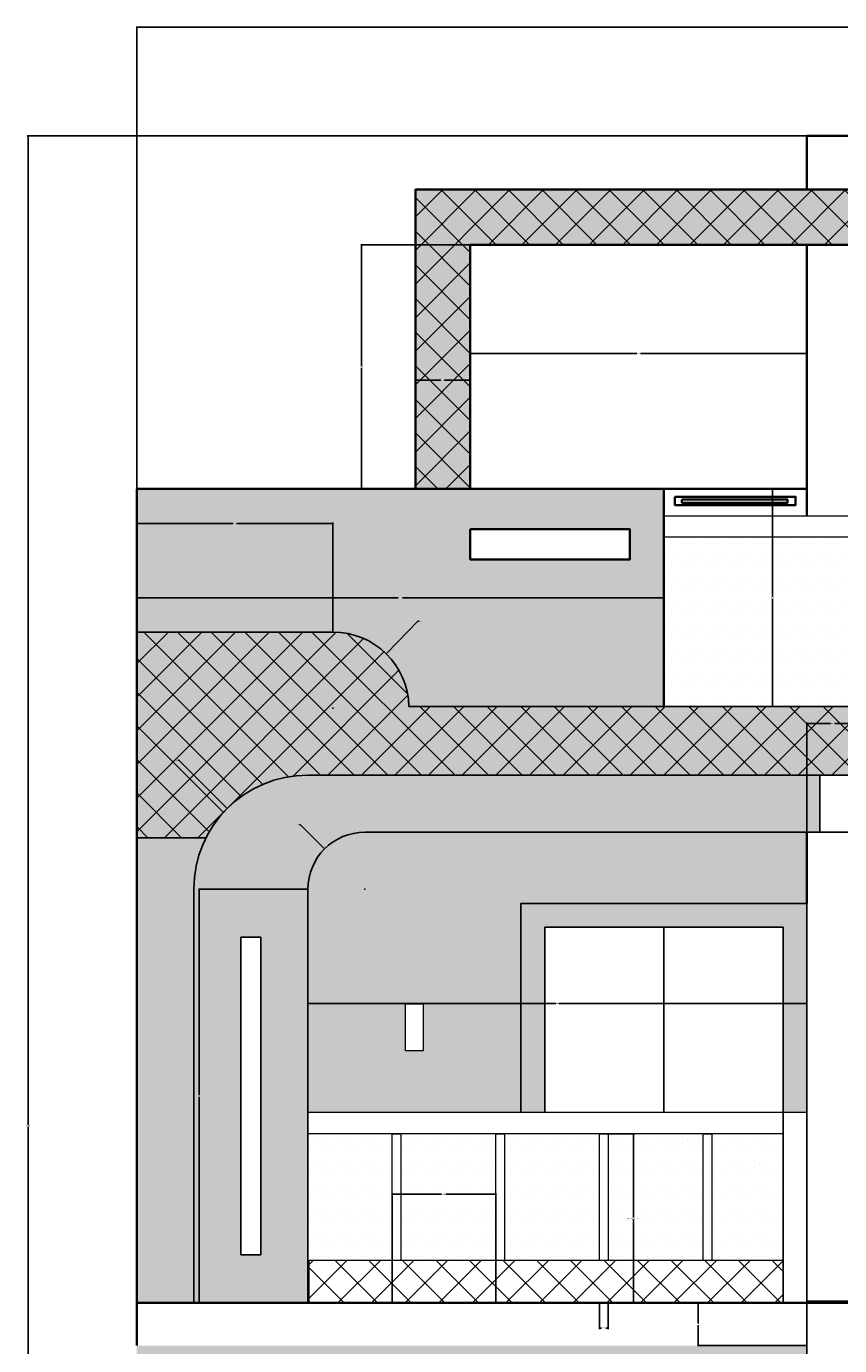
# Model space of a CAD drawing. Units: inches. Extents: x -13 to 333, y -76 to 399.
# Tile 2 of 3: x -13 to 158, y 121 to 399. Entities that reach past the tile are written whole.
import ezdxf

# ---------------------------------------------------------------- set-up
doc = ezdxf.new("R2010")
doc.units = ezdxf.units.IN
doc.header["$MEASUREMENT"] = 0
for name, color, linetype, lineweight in [('A-ANNO-DIMS', 2, 'Continuous', 18), ('A-DOOR', 3, 'Continuous', 25), ('A-ELEV-PATT', 252, 'Continuous', 13), ('A-ELEV-TRIM', 7, 'Continuous', 25), ('A-FLOR', 7, 'Continuous', 35), ('A-FLOR-HRAL', 4, 'Continuous', 20), ('A-FLOR-HRAL-PATT', 8, 'Continuous', 13), ('A-ROOF', 7, 'Continuous', 35), ('A-WALL', 7, 'Continuous', 35), ('A-WALL-PATT', 252, 'Continuous', 13), ('E-LITE-EXTR', 2, 'Continuous', 18)]:
    doc.layers.add(name, color=color, linetype=linetype, lineweight=lineweight)
doc.styles.get("Standard").update_dxf_attribs({"font": 'arial.ttf'})
doc.dimstyles.get("Standard").update_dxf_attribs({"dimtxt": 0.18, "dimasz": 0.18, "dimexe": 0.18, "dimexo": 0.0625, "dimgap": 0.09, "dimtad": 0, "dimtih": 1, "dimtoh": 1, "dimdec": 4, "dimzin": 0, "dimdsep": 46, "dimtxsty": 'Standard', "dimcen": 0.09, "dimadec": 0, "dimazin": 0, "dimtfac": 1, "dimtdec": 4, "dimtofl": 0, "dimtmove": 0, "dimatfit": 3, "dimfxl": 1, "dimtolj": 1, "dimtzin": 0, "dimarcsym": 0})

# ---------------------------------------------------------------- blocks, each defined once
blk = doc.blocks.new('LIGHT-WALL-SCONCE')
blk.add_lwpolyline([(0, 9.86), (3.7, 9.86), (3.7, 0), (0, 0)], close=True)
blk = doc.blocks.new('FASCIA-BATTEN')
blk.add_lwpolyline([(0, 12), (0, 0), (2.72, 0), (2.72, 12)])
blk = doc.blocks.new('GUARD-POST-BALCONY')
for points in [[(0, 9), (0, 35.57), (1.84, 35.57), (1.84, 9)], [(1.84, 0), (0, 0)]]:
    blk.add_lwpolyline(points)
blk = doc.blocks.new('*D12')
at = {"layer": 'A-ANNO-DIMS', "color": 0, "lineweight": -2, "transparency": 16777216}
for p, q in [((109.32, 165.75), (114.78, 165.75)), ((114.6, 165.57), (114.6, 148.15)), ((114.6, 130.36), (114.6, 147.78)), ((109.32, 130.18), (114.78, 130.18))]:
    blk.add_line(p, q, dxfattribs=at)
at = {"layer": 'A-ANNO-DIMS', "color": 0, "transparency": 16777216}
for points in [[(114.57, 165.57), (114.63, 165.57), (114.6, 165.75)], [(114.57, 130.36), (114.63, 130.36), (114.6, 130.18)]]:
    blk.add_solid(points, dxfattribs=at)
at = {"layer": 'Defpoints', "color": 0, "transparency": 16777216}
for p in [(109.26, 165.75), (114.6, 165.75), (109.26, 130.18)]:
    blk.add_point(p, dxfattribs=at)
at = {"layer": 'A-ANNO-DIMS', "color": 0, "transparency": 16777216, "insert": (114.6, 147.96), "char_height": 0.18, "attachment_point": 5}
blk.add_mtext('\\A1;BALCONY POST 36 TYP.', dxfattribs=at)
blk = doc.blocks.new('*D13')
at = {"layer": 'A-ANNO-DIMS', "color": 0, "lineweight": -2, "transparency": 16777216}
for p, q in [((107.42, 130.11), (107.42, 124.66)), ((109.26, 130.11), (109.26, 124.66)), ((107.6, 124.84), (107.88, 124.84)), ((109.08, 124.84), (108.8, 124.84))]:
    blk.add_line(p, q, dxfattribs=at)
at = {"layer": 'A-ANNO-DIMS', "color": 0, "transparency": 16777216}
for points in [[(107.6, 124.87), (107.6, 124.81), (107.42, 124.84)], [(109.08, 124.87), (109.08, 124.81), (109.26, 124.84)]]:
    blk.add_solid(points, dxfattribs=at)
at = {"layer": 'Defpoints', "color": 0, "transparency": 16777216}
for p in [(107.42, 130.18), (109.26, 130.18), (109.26, 124.84)]:
    blk.add_point(p, dxfattribs=at)
at = {"layer": 'A-ANNO-DIMS', "color": 0, "transparency": 16777216, "insert": (108.34, 124.84), "char_height": 0.18, "attachment_point": 5}
blk.add_mtext('\\A1;2 TYP.', dxfattribs=at)
blk = doc.blocks.new('*D16')
at = {"layer": 'A-ANNO-DIMS', "color": 0, "lineweight": -2, "transparency": 16777216}
for p, q in [((10.07, 301.43), (10.07, 398.67)), ((10.25, 398.49), (159.78, 398.49)), ((309.89, 398.49), (160.36, 398.49)), ((310.07, 375.69), (310.07, 398.67))]:
    blk.add_line(p, q, dxfattribs=at)
at = {"layer": 'A-ANNO-DIMS', "color": 0, "transparency": 16777216}
for points in [[(10.25, 398.52), (10.25, 398.46), (10.07, 398.49)], [(309.89, 398.52), (309.89, 398.46), (310.07, 398.49)]]:
    blk.add_solid(points, dxfattribs=at)
at = {"layer": 'Defpoints', "color": 0, "transparency": 16777216}
for p in [(310.07, 398.49), (310.07, 375.63), (10.07, 301.36)]:
    blk.add_point(p, dxfattribs=at)
at = {"layer": 'A-ANNO-DIMS', "color": 0, "transparency": 16777216, "insert": (160.07, 398.49), "char_height": 0.18, "attachment_point": 5}
blk.add_mtext('\\A1;300', dxfattribs=at)
blk = doc.blocks.new('*D17')
at = {"layer": 'A-ANNO-DIMS', "color": 0, "lineweight": -2, "transparency": 16777216}
for p, q in [((151.01, 375.63), (-12.97, 375.63)), ((-12.79, 375.45), (-12.79, 167.59)), ((-12.79, -40.64), (-12.79, 167.22)), ((10.01, -40.82), (-12.97, -40.82))]:
    blk.add_line(p, q, dxfattribs=at)
at = {"layer": 'A-ANNO-DIMS', "color": 0, "transparency": 16777216}
for points in [[(-12.82, 375.45), (-12.76, 375.45), (-12.79, 375.63)], [(-12.82, -40.64), (-12.76, -40.64), (-12.79, -40.82)]]:
    blk.add_solid(points, dxfattribs=at)
at = {"layer": 'Defpoints', "color": 0, "transparency": 16777216}
for p in [(-12.79, 375.63), (151.07, 375.63), (10.07, -40.82)]:
    blk.add_point(p, dxfattribs=at)
at = {"layer": 'A-ANNO-DIMS', "color": 0, "transparency": 16777216, "insert": (-12.79, 167.4), "char_height": 0.18, "attachment_point": 5}
blk.add_mtext('\\A1;416.46', dxfattribs=at)
blk = doc.blocks.new('*D33')
at = {"layer": 'A-ANNO-DIMS', "color": 0, "lineweight": -2, "transparency": 16777216}
for p, q in [((46.01, 217.18), (23.03, 217.18)), ((23.21, 217), (23.21, 173.86)), ((23.21, 130.36), (23.21, 173.49)), ((46.01, 130.18), (23.03, 130.18))]:
    blk.add_line(p, q, dxfattribs=at)
at = {"layer": 'A-ANNO-DIMS', "color": 0, "transparency": 16777216}
for points in [[(23.18, 217), (23.24, 217), (23.21, 217.18)], [(23.18, 130.36), (23.24, 130.36), (23.21, 130.18)]]:
    blk.add_solid(points, dxfattribs=at)
at = {"layer": 'Defpoints', "color": 0, "transparency": 16777216}
for p in [(23.21, 217.18), (46.07, 217.18), (46.07, 130.18)]:
    blk.add_point(p, dxfattribs=at)
at = {"layer": 'A-ANNO-DIMS', "color": 0, "transparency": 16777216, "insert": (23.21, 173.68), "char_height": 0.18, "attachment_point": 5}
blk.add_mtext('\\A1;87', dxfattribs=at)
blk = doc.blocks.new('*D34')
at = {"layer": 'A-ANNO-DIMS', "color": 0, "lineweight": -2, "transparency": 16777216}
for p, q in [((63.78, 130.24), (63.78, 153.22)), ((63.96, 153.04), (74.22, 153.04)), ((85.42, 153.04), (75.15, 153.04)), ((85.6, 130.24), (85.6, 153.22))]:
    blk.add_line(p, q, dxfattribs=at)
at = {"layer": 'A-ANNO-DIMS', "color": 0, "transparency": 16777216}
for points in [[(63.96, 153.07), (63.96, 153.01), (63.78, 153.04)], [(85.42, 153.07), (85.42, 153.01), (85.6, 153.04)]]:
    blk.add_solid(points, dxfattribs=at)
at = {"layer": 'Defpoints', "color": 0, "transparency": 16777216}
for p in [(85.6, 153.04), (63.78, 130.18), (85.6, 130.18)]:
    blk.add_point(p, dxfattribs=at)
at = {"layer": 'A-ANNO-DIMS', "color": 0, "transparency": 16777216, "insert": (74.69, 153.04), "char_height": 0.18, "attachment_point": 5}
blk.add_mtext('\\A1;21.823', dxfattribs=at)
blk = doc.blocks.new('*D36')
at = {"layer": 'A-ANNO-DIMS', "color": 0, "lineweight": -2, "transparency": 16777216}
for p, q in [((151.07, 229.24), (151.07, 252.22)), ((151.25, 252.04), (156.06, 252.04)), ((161.78, 252.04), (156.97, 252.04)), ((161.96, 229.24), (161.96, 252.22))]:
    blk.add_line(p, q, dxfattribs=at)
at = {"layer": 'A-ANNO-DIMS', "color": 0, "transparency": 16777216}
for points in [[(151.25, 252.07), (151.25, 252.01), (151.07, 252.04)], [(161.78, 252.07), (161.78, 252.01), (161.96, 252.04)]]:
    blk.add_solid(points, dxfattribs=at)
at = {"layer": 'Defpoints', "color": 0, "transparency": 16777216}
for p in [(161.96, 252.04), (151.07, 229.18), (161.96, 229.18)]:
    blk.add_point(p, dxfattribs=at)
at = {"layer": 'A-ANNO-DIMS', "color": 0, "transparency": 16777216, "insert": (156.51, 252.04), "char_height": 0.18, "attachment_point": 5}
blk.add_mtext('\\A1;10.885', dxfattribs=at)
blk = doc.blocks.new('*D37')
at = {"layer": 'A-ANNO-DIMS', "color": 0, "lineweight": -2, "transparency": 16777216}
for p, q in [((121.05, 301.36), (144.03, 301.36)), ((143.85, 301.18), (143.85, 278.68)), ((143.85, 255.81), (143.85, 278.32)), ((121.05, 255.63), (144.03, 255.63))]:
    blk.add_line(p, q, dxfattribs=at)
at = {"layer": 'A-ANNO-DIMS', "color": 0, "transparency": 16777216}
for points in [[(143.82, 301.18), (143.88, 301.18), (143.85, 301.36)], [(143.82, 255.81), (143.88, 255.81), (143.85, 255.63)]]:
    blk.add_solid(points, dxfattribs=at)
at = {"layer": 'Defpoints', "color": 0, "transparency": 16777216}
for p in [(120.99, 301.36), (120.99, 255.63), (143.85, 255.63)]:
    blk.add_point(p, dxfattribs=at)
at = {"layer": 'A-ANNO-DIMS', "color": 0, "transparency": 16777216, "insert": (143.85, 278.5), "char_height": 0.18, "attachment_point": 5}
blk.add_mtext('\\A1;45.73', dxfattribs=at)
blk = doc.blocks.new('*D38')
at = {"layer": 'A-ANNO-DIMS', "color": 0, "lineweight": -2, "transparency": 16777216}
for p, q in [((10.07, 301.3), (10.07, 278.32)), ((120.99, 301.3), (120.99, 278.32)), ((10.25, 278.5), (65.08, 278.5)), ((120.81, 278.5), (65.98, 278.5))]:
    blk.add_line(p, q, dxfattribs=at)
at = {"layer": 'A-ANNO-DIMS', "color": 0, "transparency": 16777216}
for points in [[(10.25, 278.53), (10.25, 278.47), (10.07, 278.5)], [(120.81, 278.53), (120.81, 278.47), (120.99, 278.5)]]:
    blk.add_solid(points, dxfattribs=at)
at = {"layer": 'Defpoints', "color": 0, "transparency": 16777216}
for p in [(10.07, 301.36), (120.99, 301.36), (10.07, 278.5)]:
    blk.add_point(p, dxfattribs=at)
at = {"layer": 'A-ANNO-DIMS', "color": 0, "transparency": 16777216, "insert": (65.53, 278.5), "char_height": 0.18, "attachment_point": 5}
blk.add_mtext('\\A1;110.92', dxfattribs=at)
blk = doc.blocks.new('*D39')
at = {"layer": 'A-ANNO-DIMS', "color": 0, "lineweight": -2, "transparency": 16777216}
for p, q in [((80.24, 352.68), (80.24, 329.71)), ((151.07, 352.68), (151.07, 329.71)), ((80.42, 329.89), (115.26, 329.89)), ((150.89, 329.89), (116.05, 329.89))]:
    blk.add_line(p, q, dxfattribs=at)
at = {"layer": 'A-ANNO-DIMS', "color": 0, "transparency": 16777216}
for points in [[(80.42, 329.92), (80.42, 329.86), (80.24, 329.89)], [(150.89, 329.92), (150.89, 329.86), (151.07, 329.89)]]:
    blk.add_solid(points, dxfattribs=at)
at = {"layer": 'Defpoints', "color": 0, "transparency": 16777216}
for p in [(80.24, 352.75), (151.07, 352.75), (80.24, 329.89)]:
    blk.add_point(p, dxfattribs=at)
at = {"layer": 'A-ANNO-DIMS', "color": 0, "transparency": 16777216, "insert": (115.65, 329.89), "char_height": 0.18, "attachment_point": 5}
blk.add_mtext('\\A1;70.83', dxfattribs=at)
blk = doc.blocks.new('*D40')
at = {"layer": 'A-ANNO-DIMS', "color": 0, "lineweight": -2, "transparency": 16777216}
for p, q in [((80.18, 352.75), (57.2, 352.75)), ((57.38, 352.57), (57.38, 327.24)), ((57.38, 301.54), (57.38, 326.87)), ((80.18, 301.36), (57.2, 301.36))]:
    blk.add_line(p, q, dxfattribs=at)
at = {"layer": 'A-ANNO-DIMS', "color": 0, "transparency": 16777216}
for points in [[(57.35, 352.57), (57.41, 352.57), (57.38, 352.75)], [(57.35, 301.54), (57.41, 301.54), (57.38, 301.36)]]:
    blk.add_solid(points, dxfattribs=at)
at = {"layer": 'Defpoints', "color": 0, "transparency": 16777216}
for p in [(57.38, 352.75), (80.24, 352.75), (80.24, 301.36)]:
    blk.add_point(p, dxfattribs=at)
at = {"layer": 'A-ANNO-DIMS', "color": 0, "transparency": 16777216, "insert": (57.38, 327.05), "char_height": 0.18, "attachment_point": 5}
blk.add_mtext('\\A1;51.38', dxfattribs=at)
blk = doc.blocks.new('*D42')
at = {"layer": 'A-ANNO-DIMS', "color": 0, "lineweight": -2, "transparency": 16777216}
for p, q in [((46.07, 170.33), (46.07, 193.31)), ((46.25, 193.13), (98.29, 193.13)), ((150.89, 193.13), (98.85, 193.13)), ((151.07, 170.33), (151.07, 193.31))]:
    blk.add_line(p, q, dxfattribs=at)
at = {"layer": 'A-ANNO-DIMS', "color": 0, "transparency": 16777216}
for points in [[(46.25, 193.16), (46.25, 193.1), (46.07, 193.13)], [(150.89, 193.16), (150.89, 193.1), (151.07, 193.13)]]:
    blk.add_solid(points, dxfattribs=at)
at = {"layer": 'Defpoints', "color": 0, "transparency": 16777216}
for p in [(151.07, 193.13), (46.07, 170.27), (151.07, 170.27)]:
    blk.add_point(p, dxfattribs=at)
at = {"layer": 'A-ANNO-DIMS', "color": 0, "transparency": 16777216, "insert": (98.57, 193.13), "char_height": 0.18, "attachment_point": 5}
blk.add_mtext('\\A1;105', dxfattribs=at)
blk = doc.blocks.new('*D43')
at = {"layer": 'A-ANNO-DIMS', "color": 0, "lineweight": -2, "transparency": 16777216}
for p, q in [((151.07, 130.11), (151.07, 107.14)), ((172.62, 130.11), (172.62, 107.14)), ((151.25, 107.32), (161.38, 107.32)), ((172.44, 107.32), (162.31, 107.32))]:
    blk.add_line(p, q, dxfattribs=at)
at = {"layer": 'A-ANNO-DIMS', "color": 0, "transparency": 16777216}
for points in [[(151.25, 107.35), (151.25, 107.29), (151.07, 107.32)], [(172.44, 107.35), (172.44, 107.29), (172.62, 107.32)]]:
    blk.add_solid(points, dxfattribs=at)
at = {"layer": 'Defpoints', "color": 0, "transparency": 16777216}
for p in [(151.07, 130.18), (172.62, 130.18), (151.07, 107.32)]:
    blk.add_point(p, dxfattribs=at)
at = {"layer": 'A-ANNO-DIMS', "color": 0, "transparency": 16777216, "insert": (161.84, 107.32), "char_height": 0.18, "attachment_point": 5}
blk.add_mtext('\\A1;21.545', dxfattribs=at)
blk = doc.blocks.new('*D46')
at = {"layer": 'A-ANNO-DIMS', "color": 0, "lineweight": -2, "transparency": 16777216}
for p, q in [((151.01, 130.18), (128.03, 130.18)), ((128.21, 130), (128.21, 125.86)), ((128.21, 121.36), (128.21, 125.49)), ((151.01, 121.18), (128.03, 121.18))]:
    blk.add_line(p, q, dxfattribs=at)
at = {"layer": 'A-ANNO-DIMS', "color": 0, "transparency": 16777216}
for points in [[(128.18, 130), (128.24, 130), (128.21, 130.18)], [(128.18, 121.36), (128.24, 121.36), (128.21, 121.18)]]:
    blk.add_solid(points, dxfattribs=at)
at = {"layer": 'Defpoints', "color": 0, "transparency": 16777216}
for p in [(128.21, 130.18), (151.07, 130.18), (151.07, 121.18)]:
    blk.add_point(p, dxfattribs=at)
at = {"layer": 'A-ANNO-DIMS', "color": 0, "transparency": 16777216, "insert": (128.21, 125.68), "char_height": 0.18, "attachment_point": 5}
blk.add_mtext('\\A1;9', dxfattribs=at)
blk = doc.blocks.new('*D47')
at = {"layer": 'A-ANNO-DIMS', "color": 0, "lineweight": -2, "transparency": 16777216}
for p, q in [((68.7, 301.43), (68.7, 324.4)), ((68.88, 324.22), (74.08, 324.22)), ((80.06, 324.22), (74.85, 324.22)), ((80.24, 301.43), (80.24, 324.4))]:
    blk.add_line(p, q, dxfattribs=at)
at = {"layer": 'A-ANNO-DIMS', "color": 0, "transparency": 16777216}
for points in [[(68.88, 324.25), (68.88, 324.19), (68.7, 324.22)], [(80.06, 324.25), (80.06, 324.19), (80.24, 324.22)]]:
    blk.add_solid(points, dxfattribs=at)
at = {"layer": 'Defpoints', "color": 0, "transparency": 16777216}
for p in [(80.24, 324.22), (68.7, 301.36), (80.24, 301.36)]:
    blk.add_point(p, dxfattribs=at)
at = {"layer": 'A-ANNO-DIMS', "color": 0, "transparency": 16777216, "insert": (74.47, 324.22), "char_height": 0.18, "attachment_point": 5}
blk.add_mtext('\\A1;11.54', dxfattribs=at)
blk = doc.blocks.new('*D50')
at = {"layer": 'A-ANNO-DIMS', "color": 0, "lineweight": -2, "transparency": 16777216}
for p, q in [((10.07, 271.33), (10.07, 294.31)), ((51.35, 271.33), (51.35, 294.31)), ((10.25, 294.13), (30.31, 294.13)), ((51.17, 294.13), (31.11, 294.13))]:
    blk.add_line(p, q, dxfattribs=at)
at = {"layer": 'A-ANNO-DIMS', "color": 0, "transparency": 16777216}
for points in [[(10.25, 294.16), (10.25, 294.1), (10.07, 294.13)], [(51.17, 294.16), (51.17, 294.1), (51.35, 294.13)]]:
    blk.add_solid(points, dxfattribs=at)
at = {"layer": 'Defpoints', "color": 0, "transparency": 16777216}
for p in [(51.35, 294.13), (10.07, 271.27), (51.35, 271.27)]:
    blk.add_point(p, dxfattribs=at)
at = {"layer": 'A-ANNO-DIMS', "color": 0, "transparency": 16777216, "insert": (30.71, 294.13), "char_height": 0.18, "attachment_point": 5}
blk.add_mtext('\\A1;41.28', dxfattribs=at)
blk = doc.blocks.new('*D51')
at = {"layer": 'A-ANNO-DIMS', "color": 0, "lineweight": -2, "transparency": 16777216}
for p, q in [((18.74, 244.33), (18.92, 244.33)), ((18.92, 244.33), (28.97, 234.27)), ((45.98, 217.18), (46.16, 217.18)), ((46.07, 217.09), (46.07, 217.27))]:
    blk.add_line(p, q, dxfattribs=at)
at = {"layer": 'A-ANNO-DIMS', "color": 0, "transparency": 16777216}
blk.add_solid([(28.99, 234.29), (28.95, 234.25), (29.1, 234.15)], dxfattribs=at)
at = {"layer": 'Defpoints', "color": 0, "transparency": 16777216}
for p in [(29.1, 234.15), (46.07, 217.18)]:
    blk.add_point(p, dxfattribs=at)
at = {"layer": 'A-ANNO-DIMS', "color": 0, "transparency": 16777216, "insert": (18.43, 244.33), "char_height": 0.18, "attachment_point": 5}
blk.add_mtext('\\A1;R24', dxfattribs=at)
blk = doc.blocks.new('*D52')
at = {"layer": 'A-ANNO-DIMS', "color": 0, "lineweight": -2, "transparency": 16777216}
for p, q in [((69.24, 273.57), (62.66, 266.84)), ((69.42, 273.57), (69.24, 273.57)), ((51.35, 255.18), (51.35, 255.36)), ((51.26, 255.27), (51.44, 255.27))]:
    blk.add_line(p, q, dxfattribs=at)
at = {"layer": 'A-ANNO-DIMS', "color": 0, "transparency": 16777216}
blk.add_solid([(62.64, 266.86), (62.68, 266.82), (62.53, 266.71)], dxfattribs=at)
at = {"layer": 'Defpoints', "color": 0, "transparency": 16777216}
for p in [(62.53, 266.71), (51.35, 255.27)]:
    blk.add_point(p, dxfattribs=at)
at = {"layer": 'A-ANNO-DIMS', "color": 0, "transparency": 16777216, "insert": (69.73, 273.57), "char_height": 0.18, "attachment_point": 5}
blk.add_mtext('\\A1;R16', dxfattribs=at)
blk = doc.blocks.new('*D53')
at = {"layer": 'A-ANNO-DIMS', "color": 0, "lineweight": -2, "transparency": 16777216}
for p, q in [((44.31, 230.75), (44.49, 230.75)), ((44.49, 230.75), (49.46, 225.79)), ((57.98, 217.18), (58.16, 217.18)), ((58.07, 217.09), (58.07, 217.27))]:
    blk.add_line(p, q, dxfattribs=at)
at = {"layer": 'A-ANNO-DIMS', "color": 0, "transparency": 16777216}
blk.add_solid([(49.48, 225.81), (49.44, 225.77), (49.59, 225.66)], dxfattribs=at)
at = {"layer": 'Defpoints', "color": 0, "transparency": 16777216}
for p in [(49.59, 225.66), (58.07, 217.18)]:
    blk.add_point(p, dxfattribs=at)
at = {"layer": 'A-ANNO-DIMS', "color": 0, "transparency": 16777216, "insert": (44.01, 230.75), "char_height": 0.18, "attachment_point": 5}
blk.add_mtext('\\A1;R12', dxfattribs=at)

msp = doc.modelspace()

# ---------------------------------------------------------------- hatches: boundary and pattern name
at = {"layer": 'A-ELEV-PATT', "transparency": 33554595}
h = msp.add_hatch(color=256, dxfattribs=at)
h.dxf.hatch_style = 1
h.set_gradient(color1=(153, 27, 30), color2=(153, 27, 30))
h.paths.add_polyline_path([(151.0707, 214.1758), (90.9079, 214.1758), (90.9079, 170.2685), (95.9079, 170.2685), (95.9079, 209.1758), (146.0707, 209.1758), (146.0707, 170.2685), (151.0707, 170.2685)])
h.paths.add_polyline_path([(151.0707, 85.1758), (90.9079, 85.1758), (90.9079, 1.1758), (95.9079, 1.1758), (95.9079, 80.1758), (146.0707, 80.1758), (146.0707, 1.1758), (151.0707, 1.1758)])
h.paths.add_polyline_path([(60.8562, 85.1758), (27.7326, 85.1758), (27.7326, 37.5603), (60.8562, 37.5603)])
h.paths.add_polyline_path([(57.8562, 82.1758), (57.8562, 40.5603), (44.2944, 40.5603), (44.2944, 82.1758)], flags=16)
h.paths.add_polyline_path([(42.6571, 82.1758), (42.6571, 40.5603), (30.7326, 40.5603), (30.7326, 82.1758)], flags=16)
at = {"layer": 'A-FLOR-HRAL-PATT'}
h = msp.add_hatch(dxfattribs=at)
h.set_pattern_fill('DOTS', color=256, scale=40, style=0)
h.paths.add_polyline_path([(120.9893, 255.6309), (161.426, 255.6309), (161.426, 291.2047), (120.9893, 291.2047)])
h.paths.add_polyline_path([(163.2631, 255.6309), (203.6999, 255.6309), (203.6999, 291.2047), (163.2631, 291.2047)], flags=0)
h.paths.add_polyline_path([(205.537, 255.6309), (245.9737, 255.6309), (245.9737, 291.2047), (205.537, 291.2047)], flags=0)
h.paths.add_polyline_path([(247.8108, 255.6309), (288.2475, 255.6309), (288.2475, 291.2047), (247.8108, 291.2047)], flags=0)
h.paths.add_polyline_path([(290.0846, 255.6309), (310.0707, 255.6309), (310.0707, 291.2047), (290.0846, 291.2047)], flags=0)
at = {"layer": 'A-FLOR-HRAL-PATT', "transparency": 33554595}
h = msp.add_hatch(dxfattribs=at)
h.set_pattern_fill('DOTS', color=256, scale=40)
h.paths.add_polyline_path([(63.778, 165.7496), (46.0707, 165.7496), (46.0707, 130.1758), (46.3341, 130.1758), (46.3341, 139.1758), (63.778, 139.1758)])
h.paths.add_polyline_path([(85.6012, 165.7496), (65.6151, 165.7496), (65.6151, 139.1758), (85.6012, 139.1758)])
h.paths.add_polyline_path([(107.4244, 165.7496), (87.4383, 165.7496), (87.4383, 139.1758), (107.4244, 139.1758)])
h.paths.add_polyline_path([(129.2475, 165.7496), (109.2615, 165.7496), (109.2615, 139.1758), (129.2475, 139.1758)])
h.paths.add_polyline_path([(146.0707, 165.7496), (131.0846, 165.7496), (131.0846, 139.1758), (146.0707, 139.1758)])
at = {"layer": 'A-FLOR-HRAL-PATT', "transparency": 33554544}
h = msp.add_hatch(dxfattribs=at)
h.set_pattern_fill('ANSI37', color=256, scale=40)
h.paths.add_polyline_path([(146.0707, 139.1758), (46.3341, 139.1758), (46.3341, 130.1758), (146.0707, 130.1758)])
at = {"layer": 'A-WALL-PATT', "transparency": 33554556}
h = msp.add_hatch(dxfattribs=at)
h.set_pattern_fill('ANSI37', color=256, scale=40)
h.paths.add_polyline_path([(51.3479, 271.2697), (10.0707, 271.2697), (10.0707, 241.1758), (10.0707, 228.0051), (24.6528, 228.0051, -0.28286751), (46.0707, 241.1758), (310.0707, 241.1758), (310.0707, 255.6309), (67.3439, 255.6309, 0.40761741)])
h.paths.add_polyline_path([(80.2381, 352.7454), (310.0707, 352.7454), (310.0707, 364.3576), (80.2381, 364.3576), (68.6976, 364.3576), (68.6976, 301.3637), (80.2381, 301.3637)])
at = {"layer": 'A-WALL-PATT', "transparency": 33554595}
h = msp.add_hatch(color=256, dxfattribs=at)
h.dxf.hatch_style = 1
h.set_gradient(color1=(175, 217, 170), color2=(175, 217, 170))
h.paths.add_polyline_path([(310.0707, 364.3576), (80.2381, 364.3576), (68.6976, 364.3576), (68.6976, 301.3637), (80.2381, 301.3637), (80.2381, 352.7454), (310.0707, 352.7454)])
h.paths.add_polyline_path([(51.3479, 271.2697), (10.0707, 271.2697), (10.0707, 241.1758), (10.0707, 228.0051), (24.6528, 228.0051, -0.28286751), (46.0707, 241.1758), (310.0707, 241.1758), (310.0707, 255.6309), (67.3439, 255.6309, 0.40761741)])
h = msp.add_hatch(color=256, dxfattribs=at)
h.dxf.hatch_style = 1
h.set_gradient(color1=(229, 232, 120), color2=(200, 201, 45), name='INVHEMISPHERICAL')
h.paths.add_polyline_path([(120.9893, 301.3637), (10.0707, 301.3637), (10.0707, 271.2697), (51.3479, 271.2697, -0.40761741), (67.3439, 255.6309), (120.9893, 255.6309)])
h.paths.add_polyline_path([(80.2381, 286.5642), (80.2381, 292.8788), (113.8366, 292.8788), (113.8366, 286.5642)], flags=16)
h = msp.add_hatch(color=256, dxfattribs=at)
h.dxf.hatch_style = 1
h.set_gradient(color1=(39, 118, 187), color2=(39, 118, 187), name='INVSPHERICAL')
h.paths.add_polyline_path([(58.0707, 229.1758), (151.0707, 229.1758), (151.0707, 241.1758), (46.0707, 241.1758, 0.41421356), (22.0707, 217.1758), (22.0707, 130.1758), (46.0707, 130.1758), (46.0707, 217.1758, -0.41421356)])
h.paths.add_polyline_path([(36.1477, 207.0573), (36.1477, 140.2942), (31.9937, 140.2942), (31.9937, 207.0573)], flags=16)
at = {"layer": 'A-WALL-PATT', "transparency": 33554531}
h = msp.add_hatch(color=256, dxfattribs=at)
h.dxf.hatch_style = 1
h.set_gradient(color1=(205, 105, 40), color2=(205, 105, 40), name='INVCURVED')
h.paths.add_polyline_path([(153.7927, 241.1758), (151.0707, 241.1758), (151.0707, 229.1758), (153.7927, 229.1758)])
h.paths.add_polyline_path([(164.6773, 241.1758), (161.9553, 241.1758), (161.9553, 229.1758), (164.6773, 229.1758)])
h.paths.add_polyline_path([(175.5619, 241.1758), (172.8398, 241.1758), (172.8398, 229.1758), (175.5619, 229.1758)])
h.paths.add_polyline_path([(186.4464, 241.1758), (183.7244, 241.1758), (183.7244, 229.1758), (186.4464, 229.1758)])
h.paths.add_polyline_path([(197.331, 241.1758), (194.609, 241.1758), (194.609, 229.1758), (197.331, 229.1758)])
h.paths.add_polyline_path([(208.2156, 241.1758), (205.4936, 241.1758), (205.4936, 229.1758), (208.2156, 229.1758)])
h.paths.add_polyline_path([(219.1001, 241.1758), (216.3781, 241.1758), (216.3781, 229.1758), (219.1001, 229.1758)])
h.paths.add_polyline_path([(229.9847, 241.1758), (227.2627, 241.1758), (227.2627, 229.1758), (229.9847, 229.1758)])
h.paths.add_polyline_path([(240.8693, 241.1758), (238.1473, 241.1758), (238.1473, 229.1758), (240.8693, 229.1758)])
h.paths.add_polyline_path([(251.7539, 241.1758), (249.0319, 241.1758), (249.0319, 229.1758), (251.7539, 229.1758)])
h.paths.add_polyline_path([(262.6384, 241.1758), (259.9164, 241.1758), (259.9164, 229.1758), (262.6384, 229.1758)])
h.paths.add_polyline_path([(273.523, 241.1758), (270.801, 241.1758), (270.801, 229.1758), (273.523, 229.1758)])
h.paths.add_polyline_path([(284.4076, 241.1758), (281.6856, 241.1758), (281.6856, 229.1758), (284.4076, 229.1758)])
h.paths.add_polyline_path([(295.2921, 241.1758), (292.5701, 241.1758), (292.5701, 229.1758), (295.2921, 229.1758)])
h.paths.add_polyline_path([(306.1767, 241.1758), (303.4547, 241.1758), (303.4547, 229.1758), (306.1767, 229.1758)])
at = {"layer": 'A-WALL-PATT', "transparency": 33554595}
h = msp.add_hatch(color=256, dxfattribs=at)
h.dxf.hatch_style = 1
h.set_gradient(color1=(255, 255, 255), name='HEMISPHERICAL')
h.paths.add_polyline_path([(22.0707, 217.1758, -0.11757059), (24.6528, 228.0051), (10.0707, 228.0051), (10.0707, 130.1758), (22.0707, 130.1758)])
h.paths.add_polyline_path([(19.0707, 112.1758), (151.0707, 112.1758), (151.0707, 121.1758), (10.0707, 121.1758), (10.0707, 1.1758), (19.0707, 1.1758)])
at = {"layer": 'A-WALL-PATT', "transparency": 33554457}
h = msp.add_hatch(color=256, dxfattribs=at)
h.dxf.hatch_style = 1
h.set_gradient(color1=(144, 237, 243), color2=(144, 237, 243), name='HEMISPHERICAL')
h.paths.add_polyline_path([(151.0707, 112.1758), (19.0707, 112.1758), (19.0707, 1.1758), (90.9079, 1.1758), (90.9079, 85.1758), (151.0707, 85.1758)])
h.paths.add_polyline_path([(60.8562, 85.1758), (60.8562, 37.5603), (27.7326, 37.5603), (27.7326, 85.1758)], flags=16)
h.paths.add_polyline_path([(57.8562, 82.1758), (57.8562, 40.5603), (44.2944, 40.5603), (44.2944, 82.1758)], flags=0)
h.paths.add_polyline_path([(70.3288, 64.0624), (70.3288, 54.1998), (66.6308, 54.1998), (66.6308, 64.0624)], flags=16)
h.paths.add_polyline_path([(42.6571, 82.1758), (42.6571, 40.5603), (30.7326, 40.5603), (30.7326, 82.1758)], flags=0)
h.paths.add_polyline_path([(90.9079, 214.1758), (151.0707, 214.1758), (151.0707, 229.1758), (58.0707, 229.1758, 0.41421356), (46.0707, 217.1758), (46.0707, 170.2685), (90.9079, 170.2685)])
h.paths.add_polyline_path([(66.6308, 193.0624), (70.3288, 193.0624), (70.3288, 183.1998), (66.6308, 183.1998)], flags=16)

# ---------------------------------------------------------------- linework, layer by layer
at = {"layer": 'A-DOOR'}
for p, q in [((146.0707, 209.1758), (95.9079, 209.1758)), ((95.9079, 209.1758), (95.9079, 170.2685)), ((120.9893, 209.1758), (120.9893, 170.2685)), ((146.0707, 130.1758), (146.0707, 209.1758))]:
    msp.add_line(p, q, dxfattribs=at)
msp.add_lwpolyline([(90.9079, 130.1758), (151.0707, 130.1758), (151.0707, 214.1758), (90.9079, 214.1758), (90.9079, 170.2685)], dxfattribs=at)
at = {"layer": 'A-ELEV-TRIM'}
for p, q in [((10.0707, 271.2697), (51.3479, 271.2697)), ((67.3439, 255.6309), (310.0707, 255.6309)), ((46.0707, 241.1758), (310.0707, 241.1758)), ((24.6528, 228.0051), (10.0707, 228.0051)), ((58.0707, 229.1758), (310.0707, 229.1758)), ((22.0707, 130.1758), (22.0707, 217.1758)), ((46.0707, 130.1758), (46.0707, 217.1758))]:
    msp.add_line(p, q, dxfattribs=at)
for points in [[(46.0707, 241.1758), (310.0707, 241.1758), (310.0707, 301.3637)], [(151.0707, 241.1758), (167.1016, 241.1758)], [(167.1016, 229.1758), (167.1016, 130.5549), (151.0707, 130.5549), (151.0707, 229.1758)]]:
    msp.add_lwpolyline(points, dxfattribs=at)
msp.add_lwpolyline([(31.9937, 140.2942), (36.1477, 140.2942), (36.1477, 207.0573), (31.9937, 207.0573)], close=True, dxfattribs=at)
for centre, radius, start, end in [((51.3479, 255.2697), 16, 1.293342, 90), ((46.0707, 217.1758), 24, 90, 180), ((58.0707, 217.1758), 12, 90, 180)]:
    msp.add_arc(centre, radius, start, end, dxfattribs=at)
at = {"layer": 'A-FLOR'}
msp.add_line((310.0707, 130.1758), (10.0707, 130.1758), dxfattribs=at)
at = {"layer": 'A-FLOR-HRAL'}
msp.add_line((146.0707, 170.2685), (151.0707, 170.2685), dxfattribs=at)
for points in [[(120.9893, 295.7236), (310.0707, 295.7236), (310.0707, 291.2047), (120.9893, 291.2047)], [(146.0707, 130.1758), (46.3341, 130.1758), (46.3341, 139.1758), (146.0707, 139.1758)]]:
    msp.add_lwpolyline(points, close=True, dxfattribs=at)
for points in [[(46.0707, 170.2685), (146.0707, 170.2685)], [(151.0707, 170.2685), (151.0707, 165.7496)], [(146.0707, 165.7496), (46.0707, 165.7496)]]:
    msp.add_lwpolyline(points, dxfattribs=at)
at = {"layer": 'A-FLOR-HRAL-PATT', "transparency": 33554556}
for p, q in [((123.5, 164.5449), (123.5, 164.5449)), ((126, 164.5449), (126, 164.5449)), ((128.5, 164.5449), (128.5, 164.5449)), ((141, 159.5449), (141, 159.5449))]:
    msp.add_line(p, q, dxfattribs=at)
at = {"layer": 'A-ROOF'}
for p, q in [((310.0707, 375.6309), (151.0707, 375.6309)), ((151.0707, 375.6309), (151.0707, 364.3576)), ((120.9893, 255.6309), (120.9893, 301.3637)), ((120.9893, 301.3637), (151.0707, 301.3637))]:
    msp.add_line(p, q, dxfattribs=at)
for points in [[(80.2381, 364.3576), (68.6976, 364.3576), (68.6976, 301.3637), (80.2381, 301.3637), (80.2381, 352.7454)], [(80.2381, 352.7454), (310.0707, 352.7454), (310.0707, 364.3576), (80.2381, 364.3576)], [(120.9893, 301.3637), (10.0707, 301.3637), (10.0707, 241.1758)]]:
    msp.add_lwpolyline(points, dxfattribs=at)
for points in [[(123.3123, 299.7323), (148.7083, 299.7323), (148.7083, 297.9743), (123.3123, 297.9743)], [(124.7859, 299.1183), (147.0009, 299.1183), (147.0009, 298.4815), (124.7859, 298.4815)], [(80.2381, 292.8788), (113.8366, 292.8788), (113.8366, 286.5642), (80.2381, 286.5642)]]:
    msp.add_lwpolyline(points, close=True, dxfattribs=at)
at = {"layer": 'A-WALL'}
for p, q in [((151.0707, 352.7454), (151.0707, 295.7236)), ((10.0707, 121.1758), (10.0707, 241.1758)), ((151.0707, 214.1758), (151.0707, 229.1758))]:
    msp.add_line(p, q, dxfattribs=at)

# ---------------------------------------------------------------- block references
at = {"layer": 'A-ELEV-TRIM'}
msp.add_blockref('FASCIA-BATTEN', (151.0707, 229.1758), dxfattribs=at)
at = {"layer": 'A-FLOR-HRAL'}
for p in [(63.778, 130.1758), (85.6012, 130.1758), (107.4244, 130.1758), (129.2475, 130.1758)]:
    msp.add_blockref('GUARD-POST-BALCONY', p, dxfattribs=at)
at = {"layer": 'E-LITE-EXTR'}
msp.add_blockref('LIGHT-WALL-SCONCE', (66.6308, 183.1998), dxfattribs=at)

# ---------------------------------------------------------------- dimensions: what is measured, and where the dimension line sits
at = {"layer": 'A-ANNO-DIMS'}
for base, p1, p2, override, picture, middle in [((310.0707, 398.4909), (10.0707, 301.3637), (310.0707, 375.6309), {"dimdec": 0, "dimlfac": 1, "dimrnd": 0, "dimzin": 0, "dimdsep": 46, "dimlunit": 2}, '*D16', (160.0707, 398.4909)), ((80.2381, 324.2237), (68.6976, 301.3637), (80.2381, 301.3637), {"dimdec": 2, "dimlfac": 1, "dimrnd": 0, "dimzin": 0, "dimdsep": 46, "dimlunit": 2}, '*D47', (74.4679, 324.2237)), ((51.3479, 294.1297), (10.0707, 271.2697), (51.3479, 271.2697), {"dimdec": 2, "dimlfac": 1, "dimrnd": 0, "dimzin": 0, "dimdsep": 46, "dimlunit": 2}, '*D50', (30.7093, 294.1297)), ((161.9553, 252.0358), (151.0707, 229.1758), (161.9553, 229.1758), {"dimdec": 3, "dimlfac": 1, "dimrnd": 0, "dimzin": 0, "dimdsep": 46, "dimlunit": 2}, '*D36', (156.513, 252.0358)), ((151.0707, 193.1285), (46.0707, 170.2685), (151.0707, 170.2685), {"dimdec": 0, "dimlfac": 1, "dimrnd": 0, "dimzin": 0, "dimdsep": 46, "dimlunit": 2}, '*D42', (98.5707, 193.1285)), ((85.6012, 153.0358), (63.778, 130.1758), (85.6012, 130.1758), {"dimdec": 3, "dimlfac": 1, "dimrnd": 0, "dimzin": 0, "dimdsep": 46, "dimlunit": 2}, '*D34', (74.6896, 153.0358))]:
    dim = msp.add_linear_dim(base=base, p1=p1, p2=p2, dimstyle='Standard', override=override, dxfattribs=at)
    dim.commit()
    dim.dimension.update_dxf_attribs({"geometry": picture, "text_midpoint": middle})
for base, p1, p2, angle, override, picture, middle in [((-12.7893, 375.6309), (10.0707, -40.8242), (151.0707, 375.6309), 90, {"dimdec": 2, "dimlfac": 1, "dimrnd": 0, "dimzin": 0, "dimdsep": 46, "dimlunit": 2}, '*D17', (-12.7893, 167.4033)), ((57.3781, 352.7454), (80.2381, 301.3637), (80.2381, 352.7454), 90, {"dimdec": 2, "dimlfac": 1, "dimrnd": 0, "dimzin": 0, "dimdsep": 46, "dimlunit": 2}, '*D40', (57.3781, 327.0545)), ((80.2381, 329.8854), (151.0707, 352.7454), (80.2381, 352.7454), 180, {"dimdec": 2, "dimlfac": 1, "dimrnd": 0, "dimzin": 0, "dimdsep": 46, "dimlunit": 2}, '*D39', (115.6544, 329.8854)), ((10.0707, 278.5037), (120.9893, 301.3637), (10.0707, 301.3637), 180, {"dimdec": 2, "dimlfac": 1, "dimrnd": 0, "dimzin": 0, "dimdsep": 46, "dimlunit": 2}, '*D38', (65.53, 278.5037)), ((143.8493, 255.6309), (120.9893, 301.3637), (120.9893, 255.6309), 270, {"dimdec": 2, "dimlfac": 1, "dimrnd": 0, "dimzin": 0, "dimdsep": 46, "dimlunit": 2}, '*D37', (143.8493, 278.4973)), ((23.2107, 217.1758), (46.0707, 130.1758), (46.0707, 217.1758), 90, {"dimdec": 0, "dimlfac": 1, "dimrnd": 0, "dimzin": 0, "dimdsep": 46, "dimlunit": 2}, '*D33', (23.2107, 173.6758)), ((128.2107, 130.1758), (151.0707, 121.1758), (151.0707, 130.1758), 90, {"dimdec": 0, "dimlfac": 1, "dimrnd": 0, "dimzin": 0, "dimdsep": 46, "dimlunit": 2}, '*D46', (128.2107, 125.6758)), ((151.0707, 107.3158), (172.6155, 130.1758), (151.0707, 130.1758), 180, {"dimdec": 3, "dimlfac": 1, "dimrnd": 0, "dimzin": 0, "dimdsep": 46, "dimlunit": 2}, '*D43', (161.8431, 107.3158))]:
    dim = msp.add_linear_dim(base=base, p1=p1, p2=p2, angle=angle, dimstyle='Standard', override=override, dxfattribs=at)
    dim.commit()
    dim.dimension.update_dxf_attribs({"geometry": picture, "text_midpoint": middle})
for center, mpoint, picture, middle in [((51.3479, 255.2697), (62.5333, 266.7103), '*D52', (69.7295, 273.5747)), ((46.0707, 217.1758), (29.0999, 234.1461), '*D51', (18.4327, 244.3283)), ((58.0707, 217.1758), (49.5852, 225.6608), '*D53', (44.0097, 230.7518))]:
    dim = msp.add_radius_dim(center=center, mpoint=mpoint, dimstyle='Standard', override={"dimdec": 0, "dimlfac": 1, "dimrnd": 0, "dimzin": 0, "dimdsep": 46, "dimlunit": 2}, dxfattribs=at)
    dim.commit()
    dim.dimension.update_dxf_attribs({"geometry": picture, "text_midpoint": middle, "dimtype": 164})
dim = msp.add_linear_dim(base=(114.5976, 165.7496), p1=(109.2615, 130.1758), p2=(109.2615, 165.7496), angle=90, text='BALCONY POST <> TYP.', dimstyle='Standard', override={"dimdec": 0, "dimlfac": 1, "dimrnd": 0, "dimzin": 0, "dimdsep": 46, "dimlunit": 2}, dxfattribs=at)
dim.commit()
dim.dimension.update_dxf_attribs({"geometry": '*D12', "text_midpoint": (114.5976, 147.9627)})
dim = msp.add_linear_dim(base=(109.2615, 124.8397), p1=(107.4244, 130.1758), p2=(109.2615, 130.1758), text='<> TYP.', dimstyle='Standard', override={"dimdec": 0, "dimlfac": 1, "dimrnd": 0, "dimzin": 0, "dimdsep": 46, "dimlunit": 2}, dxfattribs=at)
dim.commit()
dim.dimension.update_dxf_attribs({"geometry": '*D13', "text_midpoint": (108.3429, 124.8397)})

doc.saveas('drawing.dxf')
